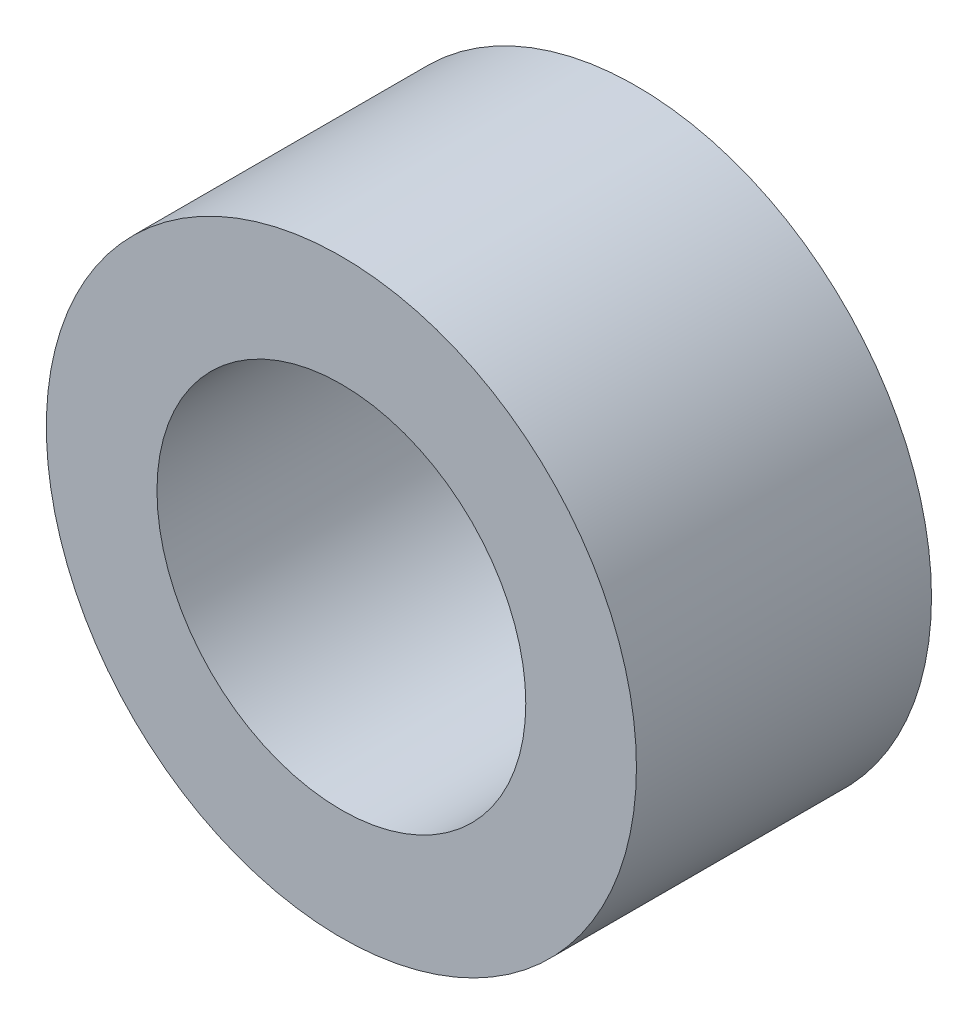
SolidWorks part; units mm, degrees
material "Plain Carbon Steel"
ref_plane "Front Plane" through (0, 0, 0) normal (0, 0, 1) x (1, 0, 0)
ref_plane "Top Plane" through (0, 0, 0) normal (0, 1, 0) x (1, 0, 0)
ref_plane "Right Plane" through (0, 0, 0) normal (1, 0, 0) x (0, 0, -1)
sketch "Bush Ring Profile Ø10 x Ø6.25" plane through (0, 0, 0) normal (0, 0, 1) x (1, 0, 0)
  circle A0 centre (0, 0) radius 3.125
  circle A1 centre (0, 0) radius 5
  dimension "D1" = 6.25
  dimension "D2" = 10
extrude "Bush Body L5" add sketch "Bush Ring Profile Ø10 x Ø6.25" along normal mid plane 5
